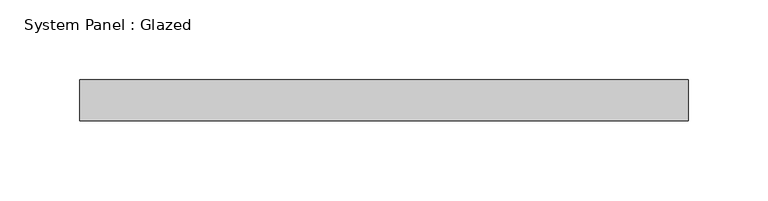
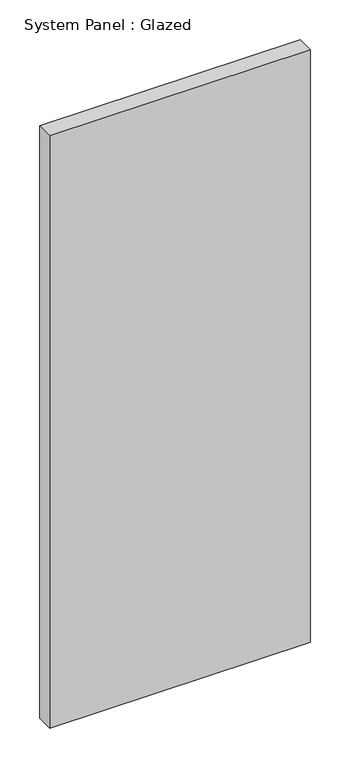
"""IFC4 building model written with IfcOpenShell, lengths in millimetres: plate geometry, System Panel : Glazed."""

from ifc_helpers import new_model, si_unit, origin, origin_with_axes, place, context, project, spatial, polyline, outline, extrude, source, transform, mapped, element, save


def system_panel_glazed_8746fe8c(model_context):
    return source(origin(), model_context, "Body", "SweptSolid", [
        extrude(outline(polyline([(190.1927764, 19.05), (-190.1927764, 19.05), (-190.1927764, 44.45), (190.1927764, 44.45), (190.1927764, 19.05)])), origin_with_axes(), (0.0, 0.0, 1.0), 914.4),
    ])


if __name__ == "__main__":
    model = new_model("IFC4")
    model_context = context("Model", 3, world=origin())
    ifc_project = project(units=[si_unit("LENGTHUNIT", "METRE", prefix="MILLI")], contexts=[model_context])
    site = spatial("IfcSite", under=ifc_project)
    building = spatial("IfcBuilding", under=site)
    placement = place(None, origin())
    system_panel_glazed_shape = system_panel_glazed_8746fe8c(model_context)
    element("IfcPlate", 1, ObjectType="System Panel : Glazed", at=placement, inside=building, context=model_context, shape_type="MappedRepresentation", body=[
        mapped(system_panel_glazed_shape, transform((0.0, 0.0, 0.0), x_axis=(1.0, 0.0, 0.0), y_axis=(0.0, 1.0, 0.0), z_axis=(0.0, 0.0, 1.0))),
    ])
    save(model, "model.ifc")

# Revit data of these elements
# Type "System Panel : Glazed"
#   Construction Type Id = "GSP4R"
#   Analytic Construction = "1/8 in Pilkington single glazing"
#   Visual Light Transmittance = 0.9
#   Solar Heat Gain Coefficient = 0.86
#   Heat Transfer Coefficient (U) = 1.18115 BTU/(h·ft²·°F)
# Element 1 (IfcPlate, "System Panel : Glazed")
#   Materials on its faces: "Glass"
# Materials
#   "Glass": class "Glass", colour RGB 0 128 192, transparency 0.75, Description = "Soda Lime Glass", Cost = 0
